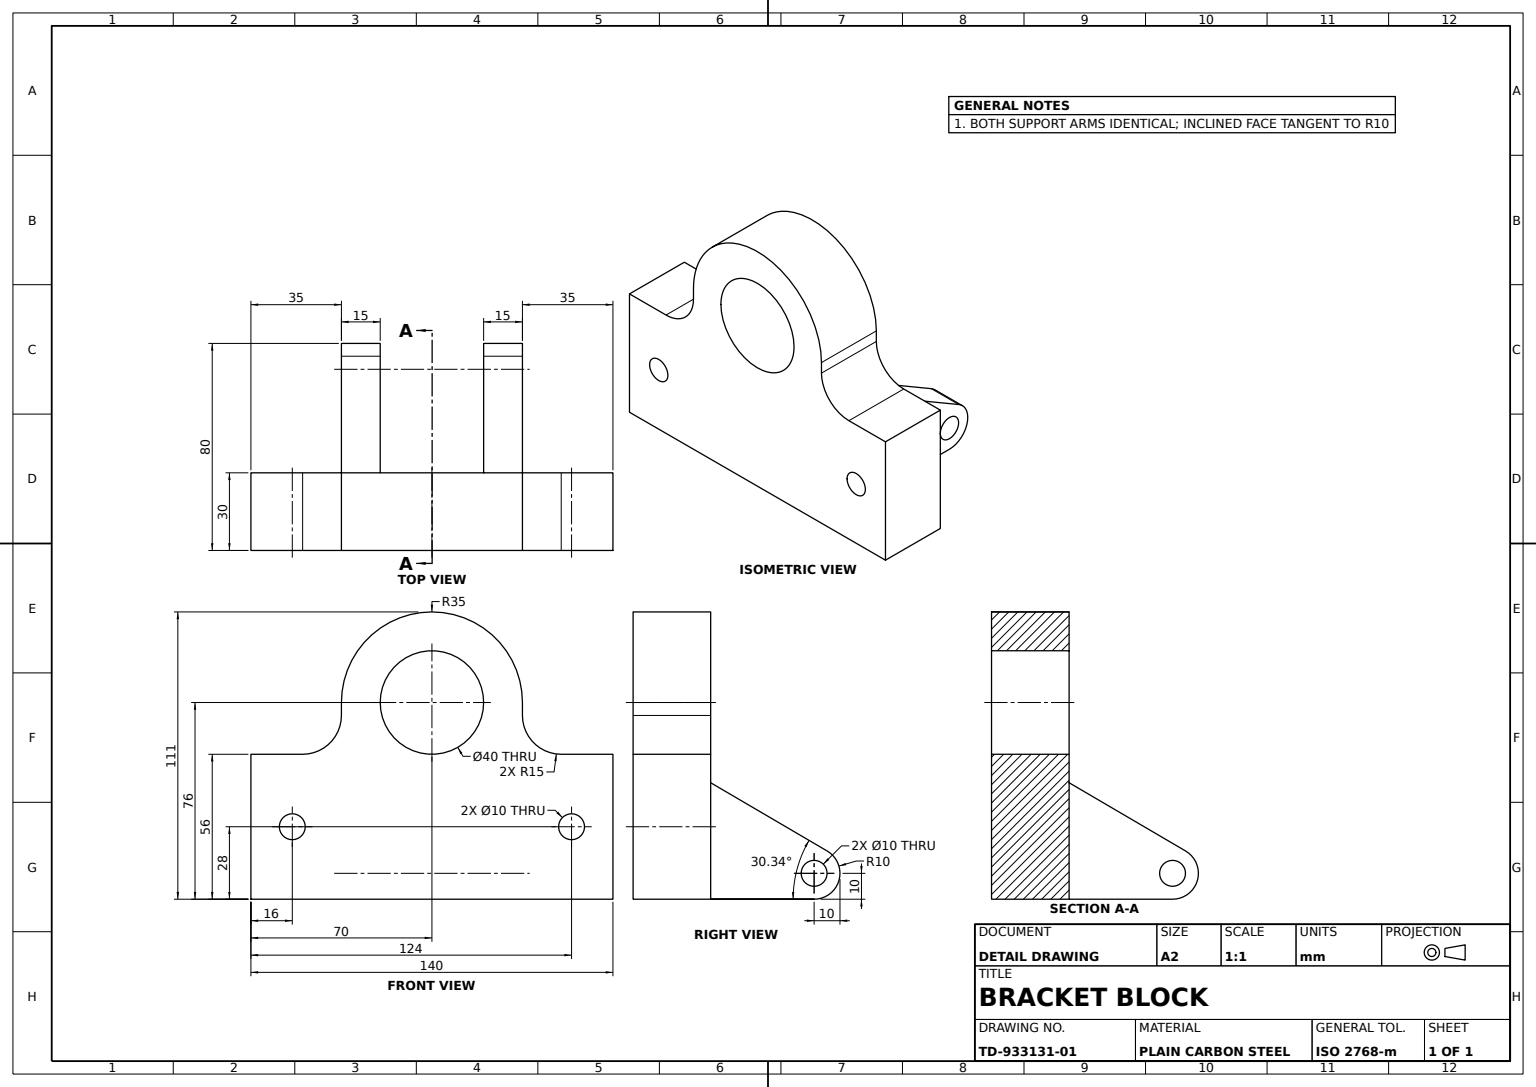
SolidWorks part; units mm, degrees
material "Plain Carbon Steel"
ref_plane "Front Plane" through (0, 0, 0) normal (0, 0, 1) x (1, 0, 0)
ref_plane "Top Plane" through (0, 0, 0) normal (0, 1, 0) x (1, 0, 0)
ref_plane "Right Plane" through (0, 0, 0) normal (1, 0, 0) x (0, 0, -1)
sketch "Base Plate Profile" plane through (0, 0, 0) normal (0, 0, 1) x (1, 0, 0)
  line L0 (0, 0) -> (0, 56)
  line L1 (0, 0) -> (140, 0)
  line L2 (140, 0) -> (140, 56)
  line L4 (0, 56) -> (20, 56)
  line L5 (140, 56) -> (125, 56)
  line L6 (125, 56) -> (120, 56)
  line L8 (105, 71) -> (105, 76)
  line L9 (35, 71) -> (35, 76)
  arc A0 (105, 76) -> (35, 76) centre (70, 76) ccw
  arc A1 (105, 71) -> (120, 56) centre (120, 71) ccw
  arc A2 (20, 56) -> (35, 71) centre (20, 71) ccw
  dimension "D1" = 140
  dimension "D2" = 35
  dimension "D3" = 15
  dimension "D4" = 35
  dimension "D5" = 56
  dimension "D7" = 125
extrude "Base Plate" add sketch "Base Plate Profile" along normal blind 30
sketch "Pivot Bore Profile" plane through (0, 0, 30) normal (0, 0, 1) x (1, 0, 0)
  circle A0 centre (70, 76) radius 20
  dimension "D1" = 40
extrude "Pivot Bore" cut sketch "Pivot Bore Profile" against normal blind 30
ref_plane "Plane1" through (35, 0, 0) normal (1, 0, 0) x (0, 0, -1)
ref_plane "Plane2" through (35, 0, 0) normal (1, 0, 0) x (0, 0, -1)
sketch "Support Arm Profile" plane through (35, 0, 0) normal (1, 0, 0) x (0, 0, -1)
  line L0 (0, 0) -> (0, 45)
  line L1 (0, 0) -> (0, 56) construction
  line L2 (0, 0) -> (40, 0)
  line L4 (0, 45) -> (45.0515, 18.6303)
  arc A0 (40, 0) -> (45.0515, 18.6303) centre (40, 10) ccw
  dimension "D1" = 10
  dimension "D2" = 40
  dimension "D3" = 45.0515
extrude "Support Arm" add sketch "Support Arm Profile" along normal blind 15
ref_plane "Plane3" through (90, 0, 0) normal (1, 0, 0) x (0, 0, -1)
sketch "Pivot Lug Profile" plane through (90, 0, 0) normal (1, 0, 0) x (0, 0, -1)
  line L0 (0, 0) -> (0, 45)
  line L1 (0, 45) -> (45.0515, 18.6303)
  line L2 (0, 0) -> (40, 0)
  arc A0 (40, 0) -> (45.0515, 18.6303) centre (40, 10) ccw
extrude "Pivot Lug" add sketch "Pivot Lug Profile" along normal blind 15
sketch "Lug Hole Profile" plane through (105, 0, 0) normal (1, 0, 0) x (0, 0, -1)
  circle A0 centre (40, 10) radius 5
  dimension "D1" = 10
extrude "Lug Hole" cut sketch "Lug Hole Profile" against normal blind 70
sketch "Mounting Holes Profile" plane through (0, 0, 0) normal (0, 0, -1) x (-1, 0, 0)
  line L0 (-105, 0) -> (-140, 0) construction
  line L1 (0, 0) -> (-35, 0) construction
  line L2 (0, 56) -> (0, 0) construction
  line L3 (-140, 0) -> (-140, 56) construction
  circle A0 centre (-124, 28) radius 5
  circle A1 centre (-16, 28) radius 5
  dimension "D1" = 28
  dimension "D5" = 10
  dimension "D6" = 10
  dimension "D2" = 28
  dimension "D3" = 16
  dimension "D4" = 16
extrude "Mounting Holes 2x" cut sketch "Mounting Holes Profile" against normal blind 70
